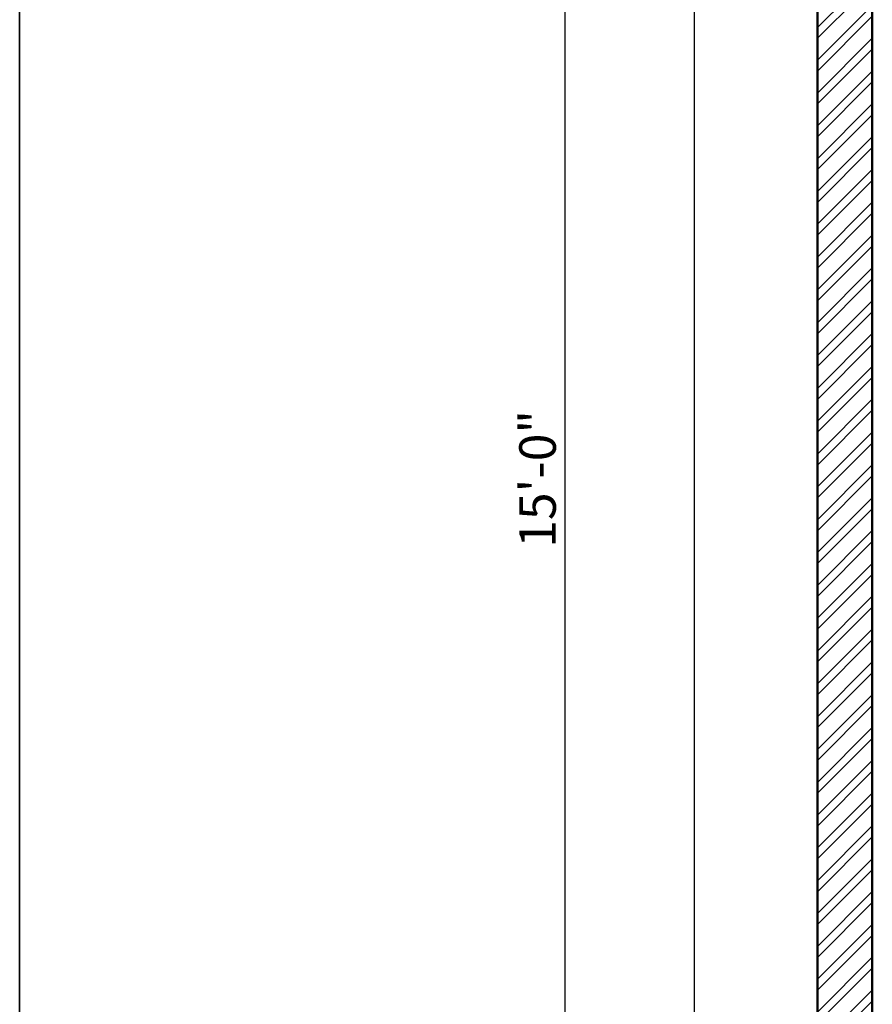
# Model space of a CAD drawing. Units: millimetres. Extents: x 20768 to 23556, y 50760 to 52704.
# Tile 9 of 36: x 20768 to 20908, y 51904 to 52066. Entities that reach past the tile are written whole.
import ezdxf

# ---------------------------------------------------------------- set-up
doc = ezdxf.new("R2010")
doc.units = ezdxf.units.MM
for name, color, linetype, lineweight in [('A-ANNO-DIMS', 2, 'Continuous', 18), ('A-ANNO-TTLB', 7, 'Continuous', 35), ('A-WALL', 7, 'Continuous', 50), ('A-WALL-PATT', 8, 'Continuous', 13), ('S-ANNO-DIMS', 2, 'Continuous', 18)]:
    doc.layers.add(name, color=color, linetype=linetype, lineweight=lineweight)
doc.styles.get("Standard").update_dxf_attribs({"font": 'arial.ttf'})
doc.dimstyles.new('ISO-25', dxfattribs={"dimtxt": 6, "dimasz": 2.5, "dimexe": 1.25, "dimexo": 0.625, "dimtad": 1, "dimdec": 0, "dimlunit": 3, "dimtxsty": 'Standard', "dimcen": 2.5, "dimadec": 0, "dimazin": 0, "dimtfac": 1, "dimtdec": 0, "dimtmove": 0, "dimatfit": 3, "dimfxl": 1, "dimarcsym": 0})

# ---------------------------------------------------------------- blocks, each defined once
blk = doc.blocks.new('*D108')
at = {"layer": 'A-ANNO-DIMS', "color": 0, "lineweight": -2, "transparency": 16777216}
for p, q in [((20898.51, 52522.9), (20877.66, 52522.9)), ((20878.91, 52520.4), (20878.91, 51832.4)), ((20898.51, 51829.9), (20877.66, 51829.9))]:
    blk.add_line(p, q, dxfattribs=at)
at = {"layer": 'A-ANNO-DIMS', "color": 0, "transparency": 16777216}
for points in [[(20878.49, 52520.4), (20879.33, 52520.4), (20878.91, 52522.9)], [(20878.49, 51832.4), (20879.33, 51832.4), (20878.91, 51829.9)]]:
    blk.add_solid(points, dxfattribs=at)
at = {"layer": 'Defpoints', "color": 0, "transparency": 16777216}
for p in [(20899.14, 52522.9), (20878.91, 51829.9), (20899.14, 51829.9)]:
    blk.add_point(p, dxfattribs=at)
at = {"layer": 'A-ANNO-DIMS', "color": 0, "transparency": 16777216, "insert": (20875.22, 52176.4), "char_height": 6, "attachment_point": 5, "rotation": 90}
blk.add_mtext('57\'-9"', dxfattribs=at)
blk = doc.blocks.new('*D204')
at = {"layer": 'Defpoints', "color": 0, "transparency": 16777216}
for p in [(20908.14, 52080.4), (20857.64, 51900.4), (20908.14, 51900.4)]:
    blk.add_point(p, dxfattribs=at)
at = {"layer": 'S-ANNO-DIMS', "color": 0, "lineweight": -2, "transparency": 16777216}
for p, q in [((20907.51, 52080.4), (20856.39, 52080.4)), ((20857.64, 52077.9), (20857.64, 51902.9)), ((20907.51, 51900.4), (20856.39, 51900.4))]:
    blk.add_line(p, q, dxfattribs=at)
at = {"layer": 'S-ANNO-DIMS', "color": 0, "transparency": 16777216}
for points in [[(20857.22, 52077.9), (20858.06, 52077.9), (20857.64, 52080.4)], [(20857.22, 51902.9), (20858.06, 51902.9), (20857.64, 51900.4)]]:
    blk.add_solid(points, dxfattribs=at)
at = {"layer": 'S-ANNO-DIMS', "color": 0, "transparency": 16777216, "insert": (20853.95, 51990.4), "char_height": 6, "attachment_point": 5, "rotation": 90}
blk.add_mtext('15\'-0"', dxfattribs=at)

msp = doc.modelspace()

# ---------------------------------------------------------------- hatches: boundary and pattern name
at = {"layer": 'A-WALL-PATT'}
h = msp.add_hatch(dxfattribs=at)
h.set_pattern_fill('ANSI32', color=256, scale=0.4)
h.set_pattern_definition([(45, (-81.1113, 0), (-2.69407684, 2.69407684), []), (45, (-79.3152, 0), (-2.69407684, 2.69407684), [])])
h.paths.add_polyline_path([(20908.14, 52077.9), (20899.14, 52077.9), (20899.14, 51902.4), (20908.14, 51902.4)])

# ---------------------------------------------------------------- linework, layer by layer
at = {"layer": 'A-ANNO-TTLB'}
msp.add_lwpolyline([(20768.14, 52703.98), (23555.8, 52703.98), (23555.8, 51623.53), (20768.14, 51623.53)], close=True, dxfattribs=at)
at = {"layer": 'A-WALL'}
for p, q in [((20899.14, 52522.9), (20899.14, 51829.9)), ((20908.14, 52513.9), (20908.14, 51838.9))]:
    msp.add_line(p, q, dxfattribs=at)

# ---------------------------------------------------------------- dimensions: what is measured, and where the dimension line sits
at = {"layer": 'A-ANNO-DIMS'}
dim = msp.add_linear_dim(base=(20878.91, 51829.9), p1=(20899.14, 52522.9), p2=(20899.14, 51829.9), angle=90, dimstyle='ISO-25', override={"dimclrd": 0, "dimclre": 0, "dimclrt": 0}, dxfattribs=at)
dim.commit()
dim.dimension.update_dxf_attribs({"geometry": '*D108', "text_midpoint": (20875.22, 52176.4)})
at = {"layer": 'S-ANNO-DIMS'}
dim = msp.add_linear_dim(base=(20857.64, 51900.4), p1=(20908.14, 52080.4), p2=(20908.14, 51900.4), angle=90, dimstyle='ISO-25', override={"dimdec": 1, "dimlfac": 1, "dimrnd": 0, "dimzin": 1, "dimdsep": 46, "dimlunit": 4, "dimfrac": 2}, dxfattribs=at)
dim.commit()
dim.dimension.update_dxf_attribs({"geometry": '*D204', "text_midpoint": (20853.95, 51990.4)})

doc.saveas('drawing.dxf')
